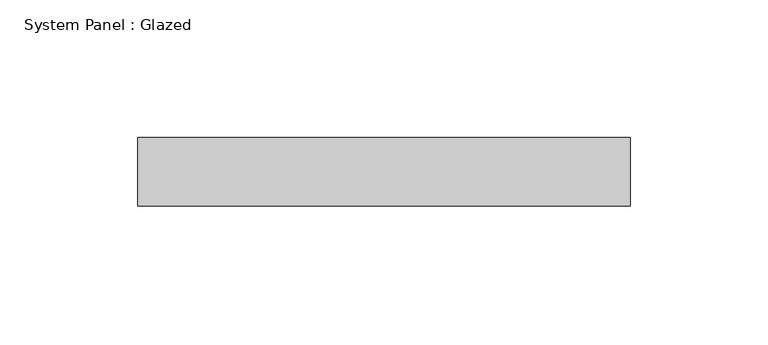
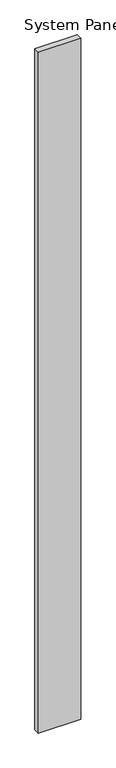
"""IFC4 building model written with IfcOpenShell, lengths in millimetres: plate geometry, System Panel : Glazed."""

from ifc_helpers import new_model, si_unit, origin, origin_with_axes, place, context, project, spatial, polyline, outline, extrude, source, transform, mapped, element, save


def system_panel_glazed_2d3c21f4(model_context):
    return source(origin(), model_context, "Body", "SweptSolid", [
        extrude(outline(polyline([(89.581546, 24.5), (-89.581546, 24.5), (-89.581546, 49.5), (89.581546, 49.5), (89.581546, 24.5)])), origin_with_axes(), (0.0, 0.0, 1.0), 3048.0),
    ])


if __name__ == "__main__":
    model = new_model("IFC4")
    model_context = context("Model", 3, world=origin())
    ifc_project = project(units=[si_unit("LENGTHUNIT", "METRE", prefix="MILLI")], contexts=[model_context])
    site = spatial("IfcSite", under=ifc_project)
    building = spatial("IfcBuilding", under=site)
    placement = place(None, origin())
    system_panel_glazed_shape = system_panel_glazed_2d3c21f4(model_context)
    element("IfcPlate", 1, ObjectType="System Panel : Glazed", at=placement, inside=building, context=model_context, shape_type="MappedRepresentation", body=[
        mapped(system_panel_glazed_shape, transform((0.0, 0.0, 0.0), x_axis=(1.0, 0.0, 0.0), y_axis=(0.0, 1.0, 0.0), z_axis=(0.0, 0.0, 1.0))),
    ])
    save(model, "model.ifc")

# Revit data of these elements
# Type "System Panel : Glazed"
#   Keynote = "H11"
#   Construction Type Id = "GSP4R"
#   Analytic Construction = "1/8 in Pilkington single glazing"
#   Visual Light Transmittance = 0.9
#   Solar Heat Gain Coefficient = 0.86
#   Heat Transfer Coefficient (U) = 6.7069 W/(m²·K)
#   Define Thermal Properties by = 1
# Element 1 (IfcPlate, "System Panel : Glazed")
#   Materials on its faces: "Glass"
# Materials
#   "Glass": class "Glass", colour RGB 0 128 192, transparency 0.9, Description = "Soda Lime Glass", Cost = 0
